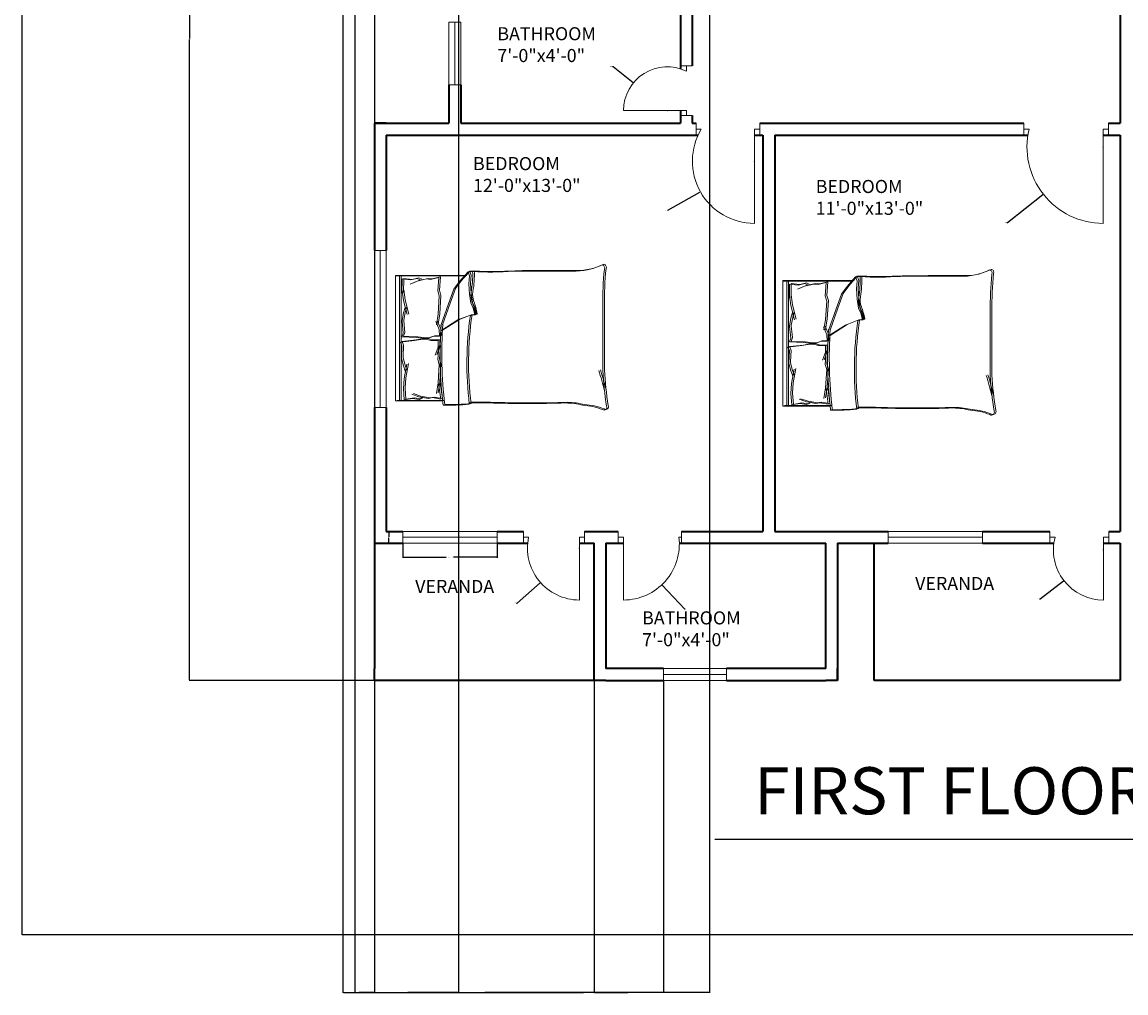
# Model space of a CAD drawing. Units: inches. Extents: x 2163 to 2982, y 1024 to 2288.
# Tile 1 of 22: x 2163 to 2585, y 1024 to 1395. Entities that reach past the tile are written whole.
import ezdxf

# ---------------------------------------------------------------- set-up
doc = ezdxf.new("R2010")
doc.units = ezdxf.units.IN
for name, color, linetype, lineweight in [('A-ANNO-DIMS', 2, 'Continuous', 18), ('A-ANNO-TTLB', 7, 'Continuous', 25), ('A-AREA-IDEN', 7, 'Continuous', 18), ('A-DOOR', 11, 'Continuous', 18), ('A-FURN', 8, 'Continuous', 13), ('A-GLAZ', 161, 'Continuous', 18), ('A-WALL', 7, 'Continuous', 35)]:
    doc.layers.add(name, color=color, linetype=linetype, lineweight=lineweight)
doc.styles.get("Standard").update_dxf_attribs({"font": 'arial.ttf'})
doc.dimstyles.get("Standard").update_dxf_attribs({"dimtxt": 0.18, "dimasz": 0.18, "dimexe": 0.18, "dimexo": 0.0625, "dimgap": 0.09, "dimtad": 0, "dimtih": 1, "dimtoh": 1, "dimdec": 4, "dimzin": 0, "dimdsep": 46, "dimtxsty": 'Standard', "dimcen": 0.09, "dimadec": 0, "dimazin": 0, "dimtfac": 1, "dimtdec": 4, "dimtofl": 0, "dimtmove": 0, "dimatfit": 3, "dimfxl": 1, "dimtolj": 1, "dimtzin": 0, "dimarcsym": 0})

# ---------------------------------------------------------------- blocks, each defined once
blk = doc.blocks.new('BED-DOUBLE')
for p, q in [((0, 51.49), (0.64, 51.49)), ((0, 3.47), (0, 51.49)), ((0, 51.27), (26.61, 51.27)), ((0, 51.27), (26.61, 51.27)), ((0.64, 51.49), (27.25, 51.49)), ((0.64, 51.49), (27.25, 51.49)), ((1.53, 3.48), (1.53, 51.27)), ((1.53, 3.47), (1.53, 51.27)), ((2.17, 3.7), (2.17, 51.49)), ((2.17, 3.7), (2.17, 51.49)), ((16.57, 50.7), (13.43, 49.92)), ((16.57, 50.7), (13.43, 49.92)), ((17.21, 50.93), (14.07, 50.15)), ((17.21, 50.93), (14.07, 50.15)), ((16.17, 45.57), (16.57, 50.7)), ((16.17, 45.57), (16.57, 50.7)), ((16.81, 45.79), (17.21, 50.93)), ((16.81, 45.79), (17.21, 50.93)), ((27.75, 52.87), (24.5, 49.16)), ((27.75, 52.87), (24.5, 49.16)), ((28.38, 53.1), (25.13, 49.39)), ((28.38, 53.1), (25.13, 49.39)), ((29.49, 52.95), (27.75, 52.87, 3.87)), ((29.49, 52.95), (27.75, 52.87, 3.87)), ((28.36, 51.33), (27.75, 52.87)), ((28.36, 51.33), (27.75, 52.87)), ((28.06, 48.23), (28.36, 51.33)), ((28.06, 48.23), (28.36, 51.33)), ((30.13, 53.18), (28.38, 53.1, 3.87)), ((29, 51.56), (28.38, 53.1)), ((30.13, 53.18), (28.38, 53.1, 3.87)), ((29, 51.56), (28.38, 53.1)), ((28.69, 48.46), (29, 51.56)), ((28.69, 48.46), (29, 51.56)), ((2.56, 50.11), (2.46, 44.71)), ((2.56, 50.11), (2.46, 44.71)), ((2.56, 50.11), (5.77, 49.73)), ((2.56, 50.11), (5.77, 49.73)), ((3.2, 50.34), (3.1, 44.94)), ((3.2, 50.34), (3.1, 44.94)), ((3.2, 50.34), (6.41, 49.96)), ((3.2, 50.34), (6.41, 49.96)), ((8.26, 49.31), (5.58, 48.13)), ((8.26, 49.31), (5.58, 48.13)), ((5.77, 49.73), (8.34, 50.33)), ((5.77, 49.73), (8.34, 50.33)), ((8.9, 49.54), (6.22, 48.36)), ((8.9, 49.54), (6.22, 48.36)), ((6.41, 49.96), (8.98, 50.56)), ((6.41, 49.96), (8.98, 50.56)), ((11.83, 50.11), (8.26, 49.31)), ((11.83, 50.11), (8.26, 49.31)), ((8.34, 50.33), (9.38, 49.81)), ((8.34, 50.33), (9.38, 49.81)), ((12.47, 50.34), (8.9, 49.54)), ((12.47, 50.34), (8.9, 49.54)), ((8.98, 50.56), (10.02, 50.04)), ((8.98, 50.56), (10.02, 50.04)), ((13.43, 49.92), (11.83, 50.11)), ((13.43, 49.92), (11.83, 50.11)), ((14.07, 50.15), (12.47, 50.34)), ((14.07, 50.15), (12.47, 50.34)), ((22.97, 46.45), (20.96, 40.87)), ((22.97, 46.45), (20.96, 40.87)), ((24.5, 49.16), (22.33, 46.22)), ((24.5, 49.16), (22.33, 46.22)), ((25.13, 49.39), (22.97, 46.45)), ((25.13, 49.39), (22.97, 46.45)), ((28.36, 44.36), (28.06, 48.23)), ((28.36, 44.36), (28.06, 48.23)), ((29, 44.59), (28.69, 48.46)), ((29, 44.59), (28.69, 48.46)), ((2.46, 44.71), (2.54, 45.71)), ((2.46, 44.71), (2.54, 45.71)), ((2.54, 45.71), (3.07, 41.91)), ((2.54, 45.71), (3.07, 41.91)), ((3.1, 44.94), (3.18, 45.94)), ((3.1, 44.94), (3.18, 45.94)), ((3.18, 45.94), (3.71, 42.14)), ((3.18, 45.94), (3.71, 42.14)), ((16.73, 43.61), (16.17, 45.57)), ((16.73, 43.61), (16.17, 45.57)), ((16.29, 36.6), (16.73, 43.61)), ((16.29, 36.6), (16.73, 43.61)), ((17.37, 43.83), (16.81, 45.79)), ((17.37, 43.83), (16.81, 45.79)), ((16.93, 36.82), (17.37, 43.83)), ((16.93, 36.82), (17.37, 43.83)), ((22.33, 46.22), (20.32, 40.64)), ((22.33, 46.22), (20.32, 40.64)), ((28.83, 40.95), (28.36, 44.36)), ((28.83, 40.95), (28.36, 44.36)), ((29.47, 41.18), (29, 44.59)), ((29.47, 41.18), (29, 44.59)), ((3.07, 41.91), (4.42, 36.49)), ((3.07, 41.91), (4.42, 36.49)), ((3.67, 39.2), (3.08, 37.14)), ((3.67, 39.2), (3.08, 37.13)), ((3.71, 42.14), (5.06, 36.72)), ((3.71, 42.14), (5.06, 36.72)), ((4.31, 39.43), (3.72, 37.36)), ((4.31, 39.43), (3.72, 37.36)), ((20.32, 40.64), (17.38, 32.31)), ((20.32, 40.64), (17.38, 32.31)), ((20.96, 40.87), (18.02, 32.53)), ((20.96, 40.87), (18.02, 32.53)), ((29.76, 38.94), (28.83, 40.95)), ((29.76, 38.94), (28.83, 40.95)), ((30.4, 39.17), (29.47, 41.18)), ((30.4, 39.17), (29.47, 41.18)), ((30.38, 36.46), (29.76, 38.94)), ((30.38, 36.46), (29.76, 38.94)), ((31.02, 36.69), (30.4, 39.17)), ((31.02, 36.69), (30.4, 39.17)), ((79.24, 15.06), (79.24, 39.68)), ((79.24, 15.06), (79.24, 39.68)), ((79.88, 15.29), (79.88, 39.91)), ((79.88, 15.29), (79.88, 39.91)), ((3.08, 37.14), (2.54, 34.2)), ((3.08, 37.13), (2.54, 34.2)), ((2.54, 34.2), (2.56, 33.88)), ((2.54, 34.2), (2.56, 33.88)), ((2.56, 33.88), (2.98, 29.46)), ((2.56, 33.88), (2.98, 29.46)), ((3.72, 37.36), (3.18, 34.43)), ((3.72, 37.36), (3.18, 34.43)), ((3.18, 34.43), (3.2, 34.11)), ((3.18, 34.43), (3.2, 34.11)), ((3.2, 34.11), (3.62, 29.68)), ((3.2, 34.11), (3.62, 29.68)), ((16.74, 30.75), (15.45, 33.82)), ((16.74, 30.75), (15.45, 33.82)), ((15.63, 32.56), (16.29, 36.6)), ((15.63, 32.56), (16.29, 36.6)), ((17.38, 30.98), (16.09, 34.05)), ((17.38, 30.98), (16.09, 34.05)), ((16.27, 32.79), (16.93, 36.82)), ((16.27, 32.79), (16.93, 36.82)), ((17.38, 30.26), (23.88, 34.45)), ((17.38, 30.26), (23.88, 34.45)), ((18.02, 30.49), (24.52, 34.68)), ((18.02, 30.49), (24.52, 34.68)), ((23.88, 34.45), (28.36, 36.15)), ((23.88, 34.45), (28.36, 36.15)), ((24.52, 34.68), (29, 36.38)), ((24.52, 34.68), (29, 36.38)), ((28.36, 36.15), (30.38, 36.46)), ((28.36, 36.15), (30.38, 36.46)), ((29, 36.38), (31.02, 36.69)), ((29, 36.38), (31.02, 36.69)), ((3.62, 29.68), (3.13, 28.21)), ((3.62, 29.68), (3.13, 28.2)), ((16.89, 28.3), (16.74, 30.75)), ((16.89, 28.3), (16.74, 30.75)), ((17.53, 28.53), (17.38, 30.98)), ((17.53, 28.53), (17.38, 30.98)), ((1.87, 25.98), (7.22, 26.56)), ((1.87, 25.98), (7.22, 26.56)), ((2.45, 24.54), (1.87, 25.98)), ((2.45, 24.54), (1.87, 25.98)), ((2.98, 29.46), (2.49, 27.98)), ((2.98, 29.46), (2.49, 27.98)), ((2.49, 27.98), (7.87, 27.73)), ((2.49, 27.98), (7.87, 27.73)), ((2.51, 26.21), (7.86, 26.79)), ((2.51, 26.21), (7.86, 26.79)), ((3.09, 24.77), (2.51, 26.21)), ((3.09, 24.77), (2.51, 26.21)), ((3.13, 28.21), (8.51, 27.96)), ((3.13, 28.2), (8.51, 27.96)), ((7.22, 26.56), (10.4, 27.14)), ((7.22, 26.56), (10.4, 27.14)), ((7.86, 26.79), (11.04, 27.37)), ((7.86, 26.79), (11.04, 27.37)), ((7.87, 27.73), (11.08, 27.35)), ((7.87, 27.73), (11.08, 27.35)), ((8.51, 27.96), (11.72, 27.58)), ((8.51, 27.96), (11.72, 27.58)), ((10.4, 27.14), (11.7, 27.14)), ((10.4, 27.14), (11.7, 27.14)), ((11.04, 27.37), (12.34, 27.37)), ((11.04, 27.37), (12.34, 27.37)), ((11.08, 27.35), (12.38, 27.44)), ((11.08, 27.35), (12.38, 27.44)), ((11.7, 27.14), (13.58, 26.56)), ((11.7, 27.14), (13.58, 26.56)), ((11.72, 27.58), (13.02, 27.66)), ((11.72, 27.58), (13.02, 27.66)), ((12.34, 27.37), (14.22, 26.79)), ((12.34, 27.37), (14.22, 26.79)), ((12.38, 27.44), (14.22, 28.13)), ((12.38, 27.44), (14.22, 28.13)), ((13.02, 27.66), (14.86, 28.36)), ((13.02, 27.66), (14.86, 28.36)), ((13.58, 26.56), (16.26, 26.56)), ((13.58, 26.56), (16.26, 26.56)), ((14.22, 28.13), (16.89, 28.3)), ((14.22, 28.13), (16.89, 28.3)), ((14.22, 26.79), (16.9, 26.79)), ((14.22, 26.79), (16.9, 26.79)), ((14.86, 28.36), (17.53, 28.53)), ((14.86, 28.36), (17.53, 28.53)), ((16.26, 26.56), (16.26, 24.1)), ((16.26, 26.56), (16.26, 24.1)), ((16.9, 26.79), (16.9, 24.33)), ((16.9, 26.79), (16.9, 24.33)), ((2.3, 20.09), (2.45, 24.54)), ((2.3, 20.09), (2.45, 24.54)), ((2.94, 20.32), (3.09, 24.77)), ((2.94, 20.32), (3.09, 24.77)), ((16.26, 24.1), (15.17, 20.96)), ((16.26, 24.1), (15.17, 20.96)), ((16.9, 24.33), (15.81, 21.19)), ((16.9, 24.33), (15.81, 21.19)), ((16.17, 19.38), (16.57, 24.52)), ((16.17, 19.38), (16.57, 24.52)), ((16.81, 19.61), (17.21, 24.74)), ((16.81, 19.61), (17.21, 24.74)), ((2.3, 19.77), (2.3, 20.09)), ((2.3, 19.77), (2.3, 20.09)), ((3.03, 16.88), (2.3, 19.77)), ((3.03, 16.88), (2.3, 19.77)), ((2.94, 20), (2.94, 20.32)), ((2.94, 20), (2.94, 20.32)), ((3.67, 17.11), (2.94, 20)), ((3.67, 17.11), (2.94, 20)), ((3.75, 14.85), (3.03, 16.88)), ((3.75, 14.85), (3.03, 16.88)), ((3.32, 12.11), (4.33, 17.6)), ((3.32, 12.11), (4.33, 17.6)), ((4.39, 15.08), (3.67, 17.11)), ((4.39, 15.08), (3.67, 17.11)), ((3.96, 12.34), (4.97, 17.83)), ((3.96, 12.34), (4.97, 17.83)), ((16.73, 17.42), (16.17, 19.38)), ((16.73, 17.42), (16.17, 19.38)), ((16.29, 10.41), (16.73, 17.42)), ((16.29, 10.41), (16.73, 17.42)), ((17.37, 17.65), (16.81, 19.61)), ((17.37, 17.65), (16.81, 19.61)), ((16.93, 10.64), (17.37, 17.65)), ((16.93, 10.64), (17.37, 17.65)), ((3.03, 8.28), (3.32, 12.11)), ((3.03, 8.28), (3.32, 12.11)), ((3.65, 8.41), (3.67, 8.51)), ((3.65, 8.41), (3.67, 8.51)), ((3.67, 8.51), (3.96, 12.34)), ((3.67, 8.51), (3.96, 12.34)), ((15.63, 6.38), (16.29, 10.41)), ((15.63, 6.38), (16.29, 10.41)), ((16.27, 6.61), (16.93, 10.64)), ((16.27, 6.61), (16.93, 10.64)), ((16.29, 10.41), (16.62, 9.28)), ((16.29, 10.41), (16.62, 9.28)), ((16.62, 9.28), (17.34, 4.18)), ((16.62, 9.28), (17.34, 4.18)), ((16.93, 10.64), (17.26, 9.51)), ((16.93, 10.64), (17.26, 9.51)), ((17.26, 9.51), (17.98, 4.41)), ((17.26, 9.51), (17.98, 4.41)), ((3.01, 8.18), (3.03, 8.28)), ((3.01, 8.18), (3.03, 8.28)), ((3.34, 3.9), (3.01, 8.18)), ((3.34, 3.9), (3.01, 8.18)), ((3.32, 3.89), (6.5, 4.47)), ((3.32, 3.89), (6.5, 4.47)), ((3.98, 4.13), (3.65, 8.41)), ((3.98, 4.13), (3.65, 8.41)), ((3.96, 4.12), (7.14, 4.7)), ((3.96, 4.12), (7.14, 4.7)), ((8.95, 5.05), (6.21, 6.06)), ((8.95, 5.05), (6.21, 6.06)), ((6.5, 4.47), (9.1, 4.04)), ((6.5, 4.47), (9.1, 4.04)), ((9.59, 5.28), (6.85, 6.29)), ((9.59, 5.28), (6.85, 6.29)), ((7.14, 4.7), (9.74, 4.27)), ((7.14, 4.7), (9.74, 4.27)), ((12.57, 4.47), (8.95, 5.05)), ((12.57, 4.47), (8.95, 5.05)), ((9.1, 4.04), (10.11, 4.62)), ((9.1, 4.04), (10.11, 4.62)), ((13.21, 4.7), (9.59, 5.28)), ((13.21, 4.7), (9.59, 5.28)), ((9.74, 4.27), (10.75, 4.85)), ((9.74, 4.27), (10.75, 4.85)), ((14.16, 4.76), (12.57, 4.47)), ((14.16, 4.76), (12.57, 4.47)), ((14.8, 4.99), (13.21, 4.7)), ((14.8, 4.99), (13.21, 4.7)), ((17.34, 4.18), (14.16, 4.76)), ((17.34, 4.18), (14.16, 4.76)), ((17.98, 4.41), (14.8, 4.99)), ((17.98, 4.41), (14.8, 4.99)), ((18.11, 3.48), (0, 3.48)), ((18.11, 3.47), (0, 3.47)), ((18.75, 3.7), (0.64, 3.7)), ((18.75, 3.7), (0.64, 3.7))]:
    blk.add_line(p, q)
for centre, radius, start, end in [((68.67, 76.16), 23.07, 267.4714, 296.4681), ((68.67, 76.16), 23.07, 267.4714, 296.4681), ((69.31, 76.39), 23.07, 267.4714, 296.4681), ((69.31, 76.39), 23.07, 267.4714, 296.4681), ((78.87, 54.41), 1.1, 332.6588, 86.02), ((78.87, 54.41), 1.1, 332.6588, 86.02), ((79.51, 54.64), 1.1, 332.6588, 86.02), ((79.51, 54.64), 1.1, 332.6588, 86.02), ((-6.66, 51.33), 36.18, 349.8763, 2.5657), ((-6.66, 51.33), 36.18, 349.8763, 2.5657), ((36.31, 182.27), 129.5, 266.9791, 273.8365), ((36.31, 182.27), 129.5, 266.9791, 273.8365), ((-6.02, 51.56), 36.18, 349.8763, 2.5657), ((-6.02, 51.56), 36.18, 349.8763, 2.5657), ((36.95, 182.49), 129.5, 266.9791, 273.8365), ((36.95, 182.49), 129.5, 266.9791, 273.8365), ((67.82, -4508.74), 4561.86, 90.00217, 90.28689), ((67.82, -4508.74), 4561.86, 90.00217, 90.28689), ((68.46, -4508.52), 4561.86, 90.00217, 90.28689), ((68.46, -4508.52), 4561.86, 90.00217, 90.28689), ((212.28, 41.15), 133.04, 174.4998, 180.6351), ((212.28, 41.15), 133.04, 174.4998, 180.6351), ((212.92, 41.38), 133.04, 174.4998, 180.6351), ((212.92, 41.38), 133.04, 174.4998, 180.6351), ((35.07, 43.74), 6.22, 168.6608, 203.7384), ((35.07, 43.74), 6.22, 168.6608, 203.7384), ((35.71, 43.97), 6.22, 168.6608, 203.7384), ((35.71, 43.97), 6.22, 168.6608, 203.7384), ((1.48, 31.15), 29.65, 10.6617, 19.8806), ((1.48, 31.15), 29.65, 10.6617, 19.8806), ((2.12, 31.38), 29.65, 10.6617, 19.8806), ((2.12, 31.38), 29.65, 10.6617, 19.8806), ((156.32, 17.76), 129.02, 171.7845, 186.9006), ((156.32, 17.76), 129.02, 171.7845, 186.9006), ((156.96, 17.98), 129.02, 171.7845, 186.9006), ((156.96, 17.98), 129.02, 171.7845, 186.9006), ((30.44, 36.64), 0.185, 250.2464, 1.1377), ((30.44, 36.64), 0.185, 250.2464, 1.1377), ((31.08, 36.86), 0.185, 250.2464, 1.1377), ((31.08, 36.86), 0.185, 250.2464, 1.1377), ((182.05, 21.36), 164.97, 176.0865, 186.7821), ((182.05, 21.36), 164.97, 176.0865, 186.7821), ((182.69, 21.59), 164.97, 176.0865, 186.7821), ((182.69, 21.59), 164.97, 176.0865, 186.7821), ((-23.71, -17.22), 106.46, 13.3832, 17.7053), ((-23.71, -17.22), 106.46, 13.3832, 17.7053), ((-23.07, -16.99), 106.46, 13.3832, 17.7053), ((-23.07, -16.99), 106.46, 13.3832, 17.7053), ((200.84, 21.43), 121.76, 182.9958, 189.4091), ((200.84, 21.43), 121.76, 182.9958, 189.4091), ((201.48, 21.66), 121.76, 182.9958, 189.4091), ((201.48, 21.65), 121.76, 182.9958, 189.4091), ((20.1, 85.16), 83.31, 268.7218, 275.604), ((20.1, 85.16), 83.31, 268.7218, 275.604), ((20.74, 85.39), 83.31, 268.7218, 275.604), ((20.74, 85.39), 83.31, 268.7218, 275.604), ((31.17, -167.31), 170.11, 88.4762, 91.0082), ((31.17, -167.31), 170.11, 88.4762, 91.0082), ((31.81, -167.08), 170.11, 88.4762, 91.0082), ((31.81, -167.08), 170.11, 88.4762, 91.0082), ((50.61, 484.82), 482.31, 268.2277, 271.7185), ((50.61, 484.82), 482.31, 268.2277, 271.7185), ((51.25, 485.05), 482.31, 268.2277, 271.7185), ((51.25, 485.05), 482.31, 268.2277, 271.7185), ((64.51, -26.9), 29.63, 76.0648, 88.9113), ((64.51, -26.9), 29.63, 76.0648, 88.9113), ((65.15, -26.67), 29.63, 76.0648, 88.9113), ((65.15, -26.67), 29.63, 76.0648, 88.9113), ((70.28, -21.66), 23.56, 67.9751, 86.652), ((70.28, -21.66), 23.56, 67.9751, 86.652), ((70.91, -21.43), 23.56, 67.9751, 86.652), ((70.91, -21.43), 23.56, 67.9751, 86.652), ((79.72, 1.09), 1.09, 236.1736, 23.4781), ((79.72, 1.09), 1.09, 236.1736, 23.4781), ((80.36, 1.32), 1.09, 236.1736, 23.4781), ((80.36, 1.32), 1.09, 236.1736, 23.4781)]:
    blk.add_arc(centre, radius, start, end)
blk = doc.blocks.new('WIN-24')
for p, q in [((0, 24), (4.5, 24)), ((0, 24), (0, 0)), ((4.5, 24), (2.25, 24)), ((2.25, 24), (2.25, 0)), ((4.5, 24), (4.5, 0)), ((2.25, 0), (0, 0)), ((0, 0), (4.5, 0))]:
    blk.add_line(p, q)
blk = doc.blocks.new('WIN-60')
for p, q in [((2.25, 60), (0, 60)), ((0, 60), (4.5, 60)), ((0, 60), (0, 0)), ((2.25, 0), (2.25, 60)), ((4.5, 60), (4.5, 0)), ((0, 0), (4.5, 0)), ((4.5, 0), (2.25, 0))]:
    blk.add_line(p, q)
blk = doc.blocks.new('WIN-36')
for p, q in [((2.25, 36), (0, 36)), ((0, 36), (4.5, 36)), ((0, 36), (0, 0)), ((2.25, 0), (2.25, 36)), ((4.5, 36), (4.5, 0)), ((0, 0), (4.5, 0)), ((4.5, 0), (2.25, 0))]:
    blk.add_line(p, q)
blk = doc.blocks.new('WIN-36-ALT')
for p, q in [((2.25, 36), (0, 36)), ((0, 36), (4.5, 36)), ((0, 36), (0, 0)), ((2.25, 0), (2.25, 36)), ((4.5, 36), (4.5, 0)), ((4.5, 0), (0, 0)), ((0, 0), (2.25, 0))]:
    blk.add_line(p, q)
blk = doc.blocks.new('*D17')
at = {"layer": 'A-ANNO-DIMS', "color": 0, "lineweight": -2, "transparency": 16777216}
for p, q in [((2308.22, 1195.71), (2308.22, 1190.19)), ((2344.22, 1195.71), (2344.22, 1190.19)), ((2308.4, 1190.37), (2324.8, 1190.37)), ((2344.04, 1190.37), (2327.64, 1190.37))]:
    blk.add_line(p, q, dxfattribs=at)
at = {"layer": 'A-ANNO-DIMS', "color": 0, "transparency": 16777216}
for points in [[(2308.4, 1190.4), (2308.4, 1190.34), (2308.22, 1190.37)], [(2344.04, 1190.4), (2344.04, 1190.34), (2344.22, 1190.37)]]:
    blk.add_solid(points, dxfattribs=at)
at = {"layer": 'Defpoints', "color": 0, "transparency": 16777216}
for p in [(2308.22, 1195.77), (2344.22, 1195.77), (2344.22, 1190.37)]:
    blk.add_point(p, dxfattribs=at)
at = {"layer": 'A-ANNO-DIMS', "color": 0, "transparency": 16777216, "insert": (2326.22, 1190.37), "char_height": 0.18, "attachment_point": 5}
blk.add_mtext('\\A1;ALT. WINDOW 36 TYP.', dxfattribs=at)
blk = doc.blocks.new('*D18')
at = {"layer": 'A-ANNO-DIMS', "color": 0, "lineweight": -2, "transparency": 16777216}
for p, q in [((2308.16, 1200.27), (2302.64, 1200.27)), ((2302.82, 1200.09), (2302.82, 1198.2)), ((2308.16, 1195.77), (2302.64, 1195.77)), ((2302.82, 1195.95), (2302.82, 1197.84))]:
    blk.add_line(p, q, dxfattribs=at)
at = {"layer": 'A-ANNO-DIMS', "color": 0, "transparency": 16777216}
for points in [[(2302.79, 1200.09), (2302.85, 1200.09), (2302.82, 1200.27)], [(2302.79, 1195.95), (2302.85, 1195.95), (2302.82, 1195.77)]]:
    blk.add_solid(points, dxfattribs=at)
at = {"layer": 'Defpoints', "color": 0, "transparency": 16777216}
for p in [(2308.22, 1200.27), (2302.82, 1195.77), (2308.22, 1195.77)]:
    blk.add_point(p, dxfattribs=at)
at = {"layer": 'A-ANNO-DIMS', "color": 0, "transparency": 16777216, "insert": (2302.82, 1198.02), "char_height": 0.18, "attachment_point": 5}
blk.add_mtext('\\A1;5 TYP.', dxfattribs=at)
blk = doc.blocks.new('*D25')
at = {"layer": 'A-ANNO-DIMS', "color": 0, "lineweight": -2, "transparency": 16777216}
for p, q in [((2297.34, 1143.21), (2297.34, 1023.79)), ((2381.34, 1143.21), (2381.34, 1023.79)), ((2297.52, 1023.97), (2339.12, 1023.97)), ((2381.16, 1023.97), (2339.56, 1023.97))]:
    blk.add_line(p, q, dxfattribs=at)
at = {"layer": 'A-ANNO-DIMS', "color": 0, "transparency": 16777216}
for points in [[(2297.52, 1024), (2297.52, 1023.94), (2297.34, 1023.97)], [(2381.16, 1024), (2381.16, 1023.94), (2381.34, 1023.97)]]:
    blk.add_solid(points, dxfattribs=at)
at = {"layer": 'Defpoints', "color": 0, "transparency": 16777216}
for p in [(2297.34, 1143.27), (2381.34, 1143.27), (2381.34, 1023.97)]:
    blk.add_point(p, dxfattribs=at)
at = {"layer": 'A-ANNO-DIMS', "color": 0, "transparency": 16777216, "insert": (2339.34, 1023.97), "char_height": 0.18, "attachment_point": 5}
blk.add_mtext('\\A1;84', dxfattribs=at)
blk = doc.blocks.new('*D26')
at = {"layer": 'A-ANNO-DIMS', "color": 0, "lineweight": -2, "transparency": 16777216}
for p, q in [((2381.34, 1143.21), (2381.34, 1023.79)), ((2407.89, 1143.21), (2407.89, 1023.79)), ((2381.52, 1023.97), (2394.22, 1023.97)), ((2407.71, 1023.97), (2395.01, 1023.97))]:
    blk.add_line(p, q, dxfattribs=at)
at = {"layer": 'A-ANNO-DIMS', "color": 0, "transparency": 16777216}
for points in [[(2381.52, 1024), (2381.52, 1023.94), (2381.34, 1023.97)], [(2407.71, 1024), (2407.71, 1023.94), (2407.89, 1023.97)]]:
    blk.add_solid(points, dxfattribs=at)
at = {"layer": 'Defpoints', "color": 0, "transparency": 16777216}
for p in [(2381.34, 1143.27), (2407.89, 1143.27), (2407.89, 1023.97)]:
    blk.add_point(p, dxfattribs=at)
at = {"layer": 'A-ANNO-DIMS', "color": 0, "transparency": 16777216, "insert": (2394.61, 1023.97), "char_height": 0.18, "attachment_point": 5}
blk.add_mtext('\\A1;26.55', dxfattribs=at)
blk = doc.blocks.new('*D30')
at = {"layer": 'A-ANNO-DIMS', "color": 0, "lineweight": -2, "transparency": 16777216}
for p, q in [((2285.34, 1633.71), (2285.34, 1023.79)), ((2297.34, 1633.71), (2297.34, 1023.79)), ((2285.52, 1023.97), (2291.13, 1023.97)), ((2297.16, 1023.97), (2291.55, 1023.97))]:
    blk.add_line(p, q, dxfattribs=at)
at = {"layer": 'A-ANNO-DIMS', "color": 0, "transparency": 16777216}
for points in [[(2285.52, 1024), (2285.52, 1023.94), (2285.34, 1023.97)], [(2297.16, 1024), (2297.16, 1023.94), (2297.34, 1023.97)]]:
    blk.add_solid(points, dxfattribs=at)
at = {"layer": 'Defpoints', "color": 0, "transparency": 16777216}
for p in [(2285.34, 1633.77), (2297.34, 1633.77), (2297.34, 1023.97)]:
    blk.add_point(p, dxfattribs=at)
at = {"layer": 'A-ANNO-DIMS', "color": 0, "transparency": 16777216, "insert": (2291.34, 1023.97), "char_height": 0.18, "attachment_point": 5}
blk.add_mtext('\\A1;12', dxfattribs=at)
blk = doc.blocks.new('*D33')
at = {"layer": 'A-ANNO-DIMS', "color": 0, "lineweight": -2, "transparency": 16777216}
for p, q in [((2285.28, 1633.77), (2226.51, 1633.77)), ((2226.69, 1633.59), (2226.69, 1388.7)), ((2226.69, 1143.45), (2226.69, 1388.34)), ((2297.28, 1143.27), (2226.51, 1143.27))]:
    blk.add_line(p, q, dxfattribs=at)
at = {"layer": 'A-ANNO-DIMS', "color": 0, "transparency": 16777216}
for points in [[(2226.66, 1633.59), (2226.72, 1633.59), (2226.69, 1633.77)], [(2226.66, 1143.45), (2226.72, 1143.45), (2226.69, 1143.27)]]:
    blk.add_solid(points, dxfattribs=at)
at = {"layer": 'Defpoints', "color": 0, "transparency": 16777216}
for p in [(2226.69, 1633.77), (2285.34, 1633.77), (2297.34, 1143.27)]:
    blk.add_point(p, dxfattribs=at)
at = {"layer": 'A-ANNO-DIMS', "color": 0, "transparency": 16777216, "insert": (2226.69, 1388.52), "char_height": 0.18, "attachment_point": 5}
blk.add_mtext('\\A1;490.5', dxfattribs=at)
blk = doc.blocks.new('*D36')
at = {"layer": 'A-ANNO-DIMS', "color": 0, "lineweight": -2, "transparency": 16777216}
for p, q in [((2289.84, 1638.21), (2289.84, 1023.79)), ((2329.44, 1638.21), (2329.44, 1023.79)), ((2290.02, 1023.97), (2309.18, 1023.97)), ((2329.26, 1023.97), (2310.11, 1023.97))]:
    blk.add_line(p, q, dxfattribs=at)
at = {"layer": 'A-ANNO-DIMS', "color": 0, "transparency": 16777216}
for points in [[(2290.02, 1024), (2290.02, 1023.94), (2289.84, 1023.97)], [(2329.26, 1024), (2329.26, 1023.94), (2329.44, 1023.97)]]:
    blk.add_solid(points, dxfattribs=at)
at = {"layer": 'Defpoints', "color": 0, "transparency": 16777216}
for p in [(2289.84, 1638.27), (2329.44, 1638.27), (2329.44, 1023.97)]:
    blk.add_point(p, dxfattribs=at)
at = {"layer": 'A-ANNO-DIMS', "color": 0, "transparency": 16777216, "insert": (2309.64, 1023.97), "char_height": 0.18, "attachment_point": 5}
blk.add_mtext('\\A1;39.605', dxfattribs=at)
blk = doc.blocks.new('*D37')
at = {"layer": 'A-ANNO-DIMS', "color": 0, "lineweight": -2, "transparency": 16777216}
for p, q in [((2329.44, 1638.21), (2329.44, 1023.79)), ((2425.44, 1638.21), (2425.44, 1023.79)), ((2329.62, 1023.97), (2377.22, 1023.97)), ((2425.26, 1023.97), (2377.66, 1023.97))]:
    blk.add_line(p, q, dxfattribs=at)
at = {"layer": 'A-ANNO-DIMS', "color": 0, "transparency": 16777216}
for points in [[(2329.62, 1024), (2329.62, 1023.94), (2329.44, 1023.97)], [(2425.26, 1024), (2425.26, 1023.94), (2425.44, 1023.97)]]:
    blk.add_solid(points, dxfattribs=at)
at = {"layer": 'Defpoints', "color": 0, "transparency": 16777216}
for p in [(2329.44, 1638.27), (2425.44, 1638.27), (2425.44, 1023.97)]:
    blk.add_point(p, dxfattribs=at)
at = {"layer": 'A-ANNO-DIMS', "color": 0, "transparency": 16777216, "insert": (2377.44, 1023.97), "char_height": 0.18, "attachment_point": 5}
blk.add_mtext('\\A1;96', dxfattribs=at)
blk = doc.blocks.new('*D42')
at = {"layer": 'A-ANNO-DIMS', "color": 0, "lineweight": -2, "transparency": 16777216}
for p, q in [((2575.85, 1347.18), (2576.03, 1347.18)), ((2575.94, 1347.09), (2575.94, 1347.27)), ((2539.28, 1318.31), (2552.88, 1329.03)), ((2539.1, 1318.31), (2539.28, 1318.31))]:
    blk.add_line(p, q, dxfattribs=at)
at = {"layer": 'A-ANNO-DIMS', "color": 0, "transparency": 16777216}
blk.add_solid([(2552.87, 1329.05), (2552.9, 1329), (2553.03, 1329.14)], dxfattribs=at)
at = {"layer": 'Defpoints', "color": 0, "transparency": 16777216}
for p in [(2575.94, 1347.18), (2553.03, 1329.14)]:
    blk.add_point(p, dxfattribs=at)
at = {"layer": 'A-ANNO-DIMS', "color": 0, "transparency": 16777216, "insert": (2538.62, 1318.31), "char_height": 0.18, "attachment_point": 5}
blk.add_mtext('\\A1;R29.16', dxfattribs=at)
blk = doc.blocks.new('*D56')
at = {"layer": 'A-ANNO-DIMS', "color": 0, "lineweight": -2, "transparency": 16777216}
for p, q in [((2442.53, 1341.76), (2442.71, 1341.76)), ((2442.62, 1341.67), (2442.62, 1341.85)), ((2409.54, 1323.08), (2421.79, 1330)), ((2409.36, 1323.08), (2409.54, 1323.08))]:
    blk.add_line(p, q, dxfattribs=at)
at = {"layer": 'A-ANNO-DIMS', "color": 0, "transparency": 16777216}
blk.add_solid([(2421.77, 1330.02), (2421.8, 1329.97), (2421.95, 1330.09)], dxfattribs=at)
at = {"layer": 'Defpoints', "color": 0, "transparency": 16777216}
for p in [(2442.62, 1341.76), (2421.95, 1330.09)]:
    blk.add_point(p, dxfattribs=at)
at = {"layer": 'A-ANNO-DIMS', "color": 0, "transparency": 16777216, "insert": (2408.88, 1323.08), "char_height": 0.18, "attachment_point": 5}
blk.add_mtext('\\A1;R23.74', dxfattribs=at)
blk = doc.blocks.new('*D63')
at = {"layer": 'A-ANNO-DIMS', "color": 0, "lineweight": -2, "transparency": 16777216}
for p, q in [((2375.6, 1193.85), (2375.78, 1193.85)), ((2375.69, 1193.76), (2375.69, 1193.94)), ((2351.9, 1172.85), (2360.69, 1180.61)), ((2351.72, 1172.85), (2351.9, 1172.85))]:
    blk.add_line(p, q, dxfattribs=at)
at = {"layer": 'A-ANNO-DIMS', "color": 0, "transparency": 16777216}
blk.add_solid([(2360.67, 1180.63), (2360.71, 1180.58), (2360.82, 1180.72)], dxfattribs=at)
at = {"layer": 'Defpoints', "color": 0, "transparency": 16777216}
for p in [(2375.69, 1193.85), (2360.82, 1180.72)]:
    blk.add_point(p, dxfattribs=at)
at = {"layer": 'A-ANNO-DIMS', "color": 0, "transparency": 16777216, "insert": (2351.17, 1172.85), "char_height": 0.18, "attachment_point": 5}
blk.add_mtext('\\A1;R19.834', dxfattribs=at)
blk = doc.blocks.new('*D64')
at = {"layer": 'A-ANNO-DIMS', "color": 0, "lineweight": -2, "transparency": 16777216}
for p, q in [((2392.47, 1195.36), (2392.65, 1195.36)), ((2392.56, 1195.27), (2392.56, 1195.45)), ((2415.95, 1170.48), (2407.3, 1179.68)), ((2416.13, 1170.48), (2415.95, 1170.48))]:
    blk.add_line(p, q, dxfattribs=at)
at = {"layer": 'A-ANNO-DIMS', "color": 0, "transparency": 16777216}
blk.add_solid([(2407.32, 1179.7), (2407.28, 1179.66), (2407.18, 1179.81)], dxfattribs=at)
at = {"layer": 'Defpoints', "color": 0, "transparency": 16777216}
for p in [(2392.56, 1195.36), (2407.18, 1179.81)]:
    blk.add_point(p, dxfattribs=at)
at = {"layer": 'A-ANNO-DIMS', "color": 0, "transparency": 16777216, "insert": (2416.68, 1170.48), "char_height": 0.18, "attachment_point": 5}
blk.add_mtext('\\A1;R21.345', dxfattribs=at)
blk = doc.blocks.new('*D65')
at = {"layer": 'A-ANNO-DIMS', "color": 0, "lineweight": -2, "transparency": 16777216}
for p, q in [((2575.97, 1193.19), (2576.15, 1193.19)), ((2576.06, 1193.1), (2576.06, 1193.28)), ((2551.79, 1174.43), (2560.75, 1181.35)), ((2551.61, 1174.43), (2551.79, 1174.43))]:
    blk.add_line(p, q, dxfattribs=at)
at = {"layer": 'A-ANNO-DIMS', "color": 0, "transparency": 16777216}
blk.add_solid([(2560.73, 1181.38), (2560.77, 1181.33), (2560.89, 1181.46)], dxfattribs=at)
at = {"layer": 'Defpoints', "color": 0, "transparency": 16777216}
for p in [(2576.06, 1193.19), (2560.89, 1181.46)]:
    blk.add_point(p, dxfattribs=at)
at = {"layer": 'A-ANNO-DIMS', "color": 0, "transparency": 16777216, "insert": (2551.13, 1174.43), "char_height": 0.18, "attachment_point": 5}
blk.add_mtext('\\A1;R19.17', dxfattribs=at)
blk = doc.blocks.new('*D74')
at = {"layer": 'A-ANNO-DIMS', "color": 0, "lineweight": -2, "transparency": 16777216}
for p, q in [((2388.37, 1378.05), (2388.55, 1378.05)), ((2388.55, 1378.05), (2396.19, 1371.85)), ((2409.19, 1361.21), (2409.37, 1361.21)), ((2409.28, 1361.12), (2409.28, 1361.3))]:
    blk.add_line(p, q, dxfattribs=at)
at = {"layer": 'A-ANNO-DIMS', "color": 0, "transparency": 16777216}
blk.add_solid([(2396.21, 1371.87), (2396.17, 1371.82), (2396.33, 1371.73)], dxfattribs=at)
at = {"layer": 'Defpoints', "color": 0, "transparency": 16777216}
for p in [(2396.33, 1371.73), (2409.28, 1361.21)]:
    blk.add_point(p, dxfattribs=at)
at = {"layer": 'A-ANNO-DIMS', "color": 0, "transparency": 16777216, "insert": (2387.82, 1378.05), "char_height": 0.18, "attachment_point": 5}
blk.add_mtext('\\A1;R16.693', dxfattribs=at)

msp = doc.modelspace()

# ---------------------------------------------------------------- linework, layer by layer
at = {"layer": 'A-ANNO-TTLB'}
msp.add_line((2427.5046, 1082.6234), (2694.9452, 1082.6234), dxfattribs=at)
msp.add_lwpolyline([(2162.6841, 2274.6054), (2982.469, 2274.6054), (2982.469, 1045.9691), (2162.6841, 1045.9691)], close=True, dxfattribs=at)
at = {"layer": 'A-DOOR'}
for p, q in [((2414.3389, 1378.2153), (2418.8389, 1378.2153)), ((2418.8389, 1378.2153), (2416.5889, 1378.2153)), ((2416.5889, 1378.2153), (2416.5889, 1376.2153)), ((2416.5889, 1361.2064), (2392.5889, 1361.2064)), ((2414.3389, 1359.2064), (2418.8389, 1359.2064)), ((2416.5889, 1359.2064), (2416.5889, 1361.2064)), ((2418.8389, 1359.2064), (2416.5889, 1359.2064)), ((2420.2902, 1356.2688), (2420.2902, 1351.7688)), ((2444.6169, 1351.7688), (2444.6169, 1356.2688)), ((2444.6169, 1356.2688), (2444.6169, 1354.0188)), ((2545.5875, 1356.2688), (2545.5875, 1351.7688)), ((2577.9364, 1356.2688), (2577.9364, 1351.7688)), ((2420.2902, 1351.7688), (2420.2902, 1354.0188)), ((2420.2902, 1354.0188), (2422.2902, 1354.0188)), ((2444.6169, 1354.0188), (2442.6169, 1354.0188)), ((2442.6169, 1354.0188), (2442.6169, 1318.0188)), ((2545.5875, 1351.7688), (2545.5875, 1354.0188)), ((2545.5875, 1354.0188), (2547.5875, 1354.0188)), ((2577.9364, 1354.0188), (2575.9364, 1354.0188)), ((2575.9364, 1354.0188), (2575.9364, 1318.0188)), ((2577.9364, 1351.7688), (2577.9364, 1354.0188)), ((2354.2961, 1195.7688), (2354.2961, 1200.2688)), ((2354.2961, 1200.2688), (2354.2961, 1198.0188)), ((2377.6878, 1195.7688), (2377.6878, 1200.2688)), ((2377.6878, 1200.2688), (2377.6878, 1198.0188)), ((2390.5578, 1195.7688), (2390.5578, 1200.2688)), ((2390.5578, 1200.2688), (2390.5578, 1198.0188)), ((2414.7365, 1200.2688), (2414.7365, 1195.7688)), ((2555.5078, 1200.2688), (2555.5078, 1195.7688)), ((2578.0618, 1200.2688), (2578.0618, 1195.7688)), ((2354.2961, 1198.0188), (2356.2961, 1198.0188)), ((2377.6878, 1198.0188), (2375.6878, 1198.0188)), ((2375.6878, 1198.0188), (2375.6878, 1174.0188)), ((2390.5578, 1198.0188), (2392.5578, 1198.0188)), ((2392.5578, 1198.0188), (2392.5578, 1174.0188)), ((2414.7365, 1198.0188), (2413.7365, 1198.0188)), ((2414.7365, 1195.7688), (2414.7365, 1198.0188)), ((2555.5078, 1195.7688), (2555.5078, 1198.0188)), ((2555.5078, 1198.0188), (2557.5078, 1198.0188)), ((2578.0618, 1198.0188), (2576.0618, 1198.0188)), ((2576.0618, 1198.0188), (2576.0618, 1174.0188)), ((2578.0618, 1195.7688), (2578.0618, 1198.0188))]:
    msp.add_line(p, q, dxfattribs=at)
for centre, radius, start, end in [((2409.282, 1361.2064), 16.693, 64.041202, 180), ((2442.6169, 1341.7574), 23.7385, 148.900687, 270), ((2575.9364, 1347.1808), 29.162, 166.438836, 270), ((2375.6878, 1193.8529), 19.8341, 167.875456, 270), ((2392.5578, 1195.3634), 21.3445, 270, 7.146709), ((2576.0618, 1193.1907), 19.1719, 165.413883, 270)]:
    msp.add_arc(centre, radius, start, end, dxfattribs=at)
at = {"layer": 'A-WALL'}
for p, q in [((2582.3389, 1633.7688), (2582.3389, 1356.2688)), ((2414.3389, 1408.7688), (2414.3389, 1377.1151)), ((2418.8389, 1408.7688), (2418.8389, 1378.2153)), ((2325.8389, 1370.9788), (2325.8389, 1356.2688)), ((2330.3389, 1370.9788), (2330.3389, 1356.2688)), ((2414.3389, 1361.2064), (2414.3389, 1356.2688)), ((2418.8389, 1359.2064), (2418.8389, 1356.2688)), ((2297.3389, 1356.2688), (2325.8389, 1356.2688)), ((2297.3389, 1356.2688), (2297.3389, 1307.663)), ((2301.8389, 1356.2688), (2297.3389, 1356.2688)), ((2297.3389, 1356.2688), (2297.3389, 1351.7688)), ((2330.3389, 1356.2688), (2414.3389, 1356.2688)), ((2418.8389, 1356.2688), (2420.2902, 1356.2688)), ((2444.6169, 1356.2688), (2545.5875, 1356.2688)), ((2577.9364, 1356.2688), (2582.3389, 1356.2688)), ((2301.8389, 1351.7688), (2301.8389, 1307.663)), ((2301.8389, 1351.7688), (2421.0927, 1351.7688)), ((2442.6169, 1351.7688), (2445.8389, 1351.7688)), ((2445.8389, 1351.7688), (2445.8389, 1200.2688)), ((2450.3389, 1351.7688), (2450.3389, 1200.2688)), ((2450.3389, 1351.7688), (2547.1376, 1351.7688)), ((2575.9364, 1351.7688), (2582.3389, 1351.7688)), ((2582.3389, 1351.7688), (2582.3389, 1200.2688)), ((2297.3389, 1247.663), (2297.3389, 1195.7688)), ((2301.8389, 1247.663), (2301.8389, 1200.2688)), ((2301.8389, 1200.2688), (2308.2199, 1200.2688)), ((2344.2199, 1200.2688), (2354.2961, 1200.2688)), ((2377.6878, 1200.2688), (2390.5578, 1200.2688)), ((2414.7365, 1200.2688), (2445.8389, 1200.2688)), ((2450.3389, 1200.2688), (2493.7336, 1200.2688)), ((2529.7336, 1200.2688), (2555.5078, 1200.2688)), ((2578.0618, 1200.2688), (2582.3389, 1200.2688)), ((2297.3389, 1195.7688), (2308.2199, 1195.7688)), ((2297.3389, 1195.7688), (2297.3389, 1147.7688)), ((2344.2199, 1195.7688), (2355.9464, 1195.7688)), ((2375.6878, 1195.7688), (2381.3389, 1195.7688)), ((2381.3389, 1143.2688), (2381.3389, 1195.7688)), ((2385.8389, 1195.7688), (2385.8389, 1147.7688)), ((2385.8389, 1195.7688), (2392.5578, 1195.7688)), ((2413.8984, 1195.7688), (2469.8389, 1195.7688)), ((2469.8389, 1147.7688), (2469.8389, 1195.7688)), ((2474.3389, 1195.7688), (2474.3389, 1143.2688)), ((2474.3389, 1195.7688), (2493.7336, 1195.7688)), ((2488.3425, 1143.2688), (2488.3425, 1195.7688)), ((2529.7336, 1195.7688), (2557.0641, 1195.7688)), ((2576.0618, 1195.7688), (2582.3389, 1195.7688)), ((2582.3389, 1195.7688), (2582.3389, 1147.7688)), ((2297.3389, 1143.2688), (2297.3389, 1147.7688)), ((2407.8903, 1147.7688), (2385.8389, 1147.7688)), ((2469.8389, 1147.7688), (2431.8903, 1147.7688)), ((2474.3389, 1143.2688), (2474.3389, 1147.7688)), ((2582.3389, 1147.7688), (2582.3389, 1143.2688)), ((2385.8389, 1143.2688), (2297.3389, 1143.2688)), ((2385.8389, 1143.2688), (2407.8903, 1143.2688)), ((2431.8903, 1143.2688), (2469.8389, 1143.2688)), ((2474.3389, 1143.2688), (2469.8389, 1143.2688)), ((2582.3389, 1143.2688), (2488.3425, 1143.2688))]:
    msp.add_line(p, q, dxfattribs=at)

# ---------------------------------------------------------------- block references
at = {"layer": 'A-FURN'}
for p in [(2305.3958, 1246.6393), (2453.4956, 1244.7033)]:
    msp.add_blockref('BED-DOUBLE', p, dxfattribs=at)
at = {"layer": 'A-GLAZ', "extrusion": (0, 0, -1), "zscale": -1}
for p, rotation in [((-2325.839, 1394.9784), 180), ((-2407.8907, 1143.2689), 90)]:
    msp.add_blockref('WIN-24', p, dxfattribs=dict(at, rotation=rotation))
at = {"layer": 'A-GLAZ'}
msp.add_blockref('WIN-60', (2297.339, 1247.6629), dxfattribs=at)
at = {"layer": 'A-GLAZ', "rotation": 270}
for name, p in [('WIN-36-ALT', (2308.2204, 1200.2688)), ('WIN-36', (2493.7332, 1200.2688))]:
    msp.add_blockref(name, p, dxfattribs=at)

# ---------------------------------------------------------------- texts
at = {"layer": 'A-ANNO-TTLB', "insert": (2442.4425, 1110.0829), "char_height": 18, "attachment_point": 1}
msp.add_mtext_dynamic_manual_height_columns('FIRST FLOOR PLAN', width=728.99492, gutter_width=12.5, heights=[0], dxfattribs=at)
at = {"layer": 'A-AREA-IDEN', "char_height": 5, "attachment_point": 1}
for s, width, insert in [('BATHROOM\\P7\'-0"x4\'-0"', 49.988909, (2344.3398, 1393.02)), ('BEDROOM\\P12\'-0"x13\'-0"', 72.064402, (2335.0379, 1343.3626)), ('BEDROOM\\P11\'-0"x13\'-0"', 58.429861, (2466.0168, 1334.6184)), ('VERANDA', 45.397901, (2312.9401, 1181.6992)), ('VERANDA', 72.810048, (2504.0273, 1182.8344)), ('BATHROOM\\P7\'-0"x4\'-0"', 41.488634, (2399.6605, 1169.6791))]:
    msp.add_mtext_dynamic_manual_height_columns(s, width=width, gutter_width=12.5, heights=[0], dxfattribs=dict(at, insert=insert))

# ---------------------------------------------------------------- dimensions: what is measured, and where the dimension line sits
at = {"layer": 'A-ANNO-DIMS'}
for base, p1, p2, override, picture, middle in [((2329.44344, 1023.97342), (2289.83891, 1638.26884), (2329.44344, 1638.26884), {"dimdec": 3, "dimlfac": 1, "dimrnd": 0, "dimzin": 0, "dimdsep": 46, "dimlunit": 2}, '*D36', (2309.64118, 1023.97342)), ((2425.4434, 1023.9734), (2329.4434, 1638.2688), (2425.4434, 1638.2688), {"dimdec": 0, "dimlfac": 1, "dimrnd": 0, "dimzin": 0, "dimdsep": 46, "dimlunit": 2}, '*D37', (2377.4434, 1023.9734)), ((2297.3389, 1023.9734), (2285.3389, 1633.7688), (2297.3389, 1633.7688), {"dimdec": 0, "dimlfac": 1, "dimrnd": 0, "dimzin": 0, "dimdsep": 46, "dimlunit": 2}, '*D30', (2291.3389, 1023.9734)), ((2381.3389, 1023.9734), (2297.3389, 1143.2688), (2381.3389, 1143.2688), {"dimdec": 0, "dimlfac": 1, "dimrnd": 0, "dimzin": 0, "dimdsep": 46, "dimlunit": 2}, '*D25', (2339.3389, 1023.9734)), ((2407.8903, 1023.9734), (2381.3389, 1143.2688), (2407.8903, 1143.2688), {"dimdec": 2, "dimlfac": 1, "dimrnd": 0, "dimzin": 0, "dimdsep": 46, "dimlunit": 2}, '*D26', (2394.6146, 1023.9734))]:
    dim = msp.add_linear_dim(base=base, p1=p1, p2=p2, dimstyle='Standard', override=override, dxfattribs=at)
    dim.commit()
    dim.dimension.update_dxf_attribs({"geometry": picture, "text_midpoint": middle})
dim = msp.add_linear_dim(base=(2226.6889, 1633.7688), p1=(2297.3389, 1143.2688), p2=(2285.3389, 1633.7688), angle=90, dimstyle='Standard', override={"dimdec": 1, "dimlfac": 1, "dimrnd": 0, "dimzin": 0, "dimdsep": 46, "dimlunit": 2}, dxfattribs=at)
dim.commit()
dim.dimension.update_dxf_attribs({"geometry": '*D33', "text_midpoint": (2226.6889, 1388.5188)})
for center, mpoint, override, picture, middle in [((2409.282, 1361.2064), (2396.3272, 1371.7341), {"dimdec": 3, "dimlfac": 1, "dimrnd": 0, "dimzin": 0, "dimdsep": 46, "dimlunit": 2}, '*D74', (2387.8246, 1378.0507)), ((2575.9364, 1347.1808), (2553.0253, 1329.1392), {"dimdec": 2, "dimlfac": 1, "dimrnd": 0, "dimzin": 0, "dimdsep": 46, "dimlunit": 2}, '*D42', (2538.6188, 1318.3142)), ((2442.6169, 1341.7574), (2421.9458, 1330.0859), {"dimdec": 2, "dimlfac": 1, "dimrnd": 0, "dimzin": 0, "dimdsep": 46, "dimlunit": 2}, '*D56', (2408.8837, 1323.083)), ((2392.5578, 1195.3634), (2407.1772, 1179.8115), {"dimdec": 3, "dimlfac": 1, "dimrnd": 0, "dimzin": 0, "dimdsep": 46, "dimlunit": 2}, '*D64', (2416.6793, 1170.4804)), ((2375.6878, 1193.8529), (2360.8205, 1180.7245), {"dimdec": 3, "dimlfac": 1, "dimrnd": 0, "dimzin": 0, "dimdsep": 46, "dimlunit": 2}, '*D63', (2351.1707, 1172.8475)), ((2576.0618, 1193.1907), (2560.8942, 1181.4644), {"dimdec": 2, "dimlfac": 1, "dimrnd": 0, "dimzin": 0, "dimdsep": 46, "dimlunit": 2}, '*D65', (2551.1338, 1174.4287))]:
    dim = msp.add_radius_dim(center=center, mpoint=mpoint, dimstyle='Standard', override=override, dxfattribs=at)
    dim.commit()
    dim.dimension.update_dxf_attribs({"geometry": picture, "text_midpoint": middle, "dimtype": 164})
dim = msp.add_linear_dim(base=(2302.8198992483, 1195.7688407479), p1=(2308.2198992483, 1200.2688407479), p2=(2308.2198992483, 1195.7688407479), angle=270, text='<> TYP.', dimstyle='Standard', override={"dimdec": 0, "dimlfac": 1, "dimrnd": 0, "dimzin": 0, "dimdsep": 46, "dimlunit": 2}, dxfattribs=at)
dim.commit()
dim.dimension.update_dxf_attribs({"geometry": '*D18', "text_midpoint": (2302.8198992483, 1198.0188407479)})
dim = msp.add_linear_dim(base=(2344.2199, 1190.3688), p1=(2308.2199, 1195.7688), p2=(2344.2199, 1195.7688), text='ALT. WINDOW <> TYP.', dimstyle='Standard', override={"dimdec": 0, "dimlfac": 1, "dimrnd": 0, "dimzin": 0, "dimdsep": 46, "dimlunit": 2}, dxfattribs=at)
dim.commit()
dim.dimension.update_dxf_attribs({"geometry": '*D17', "text_midpoint": (2326.2199, 1190.3688)})

doc.saveas('drawing.dxf')
